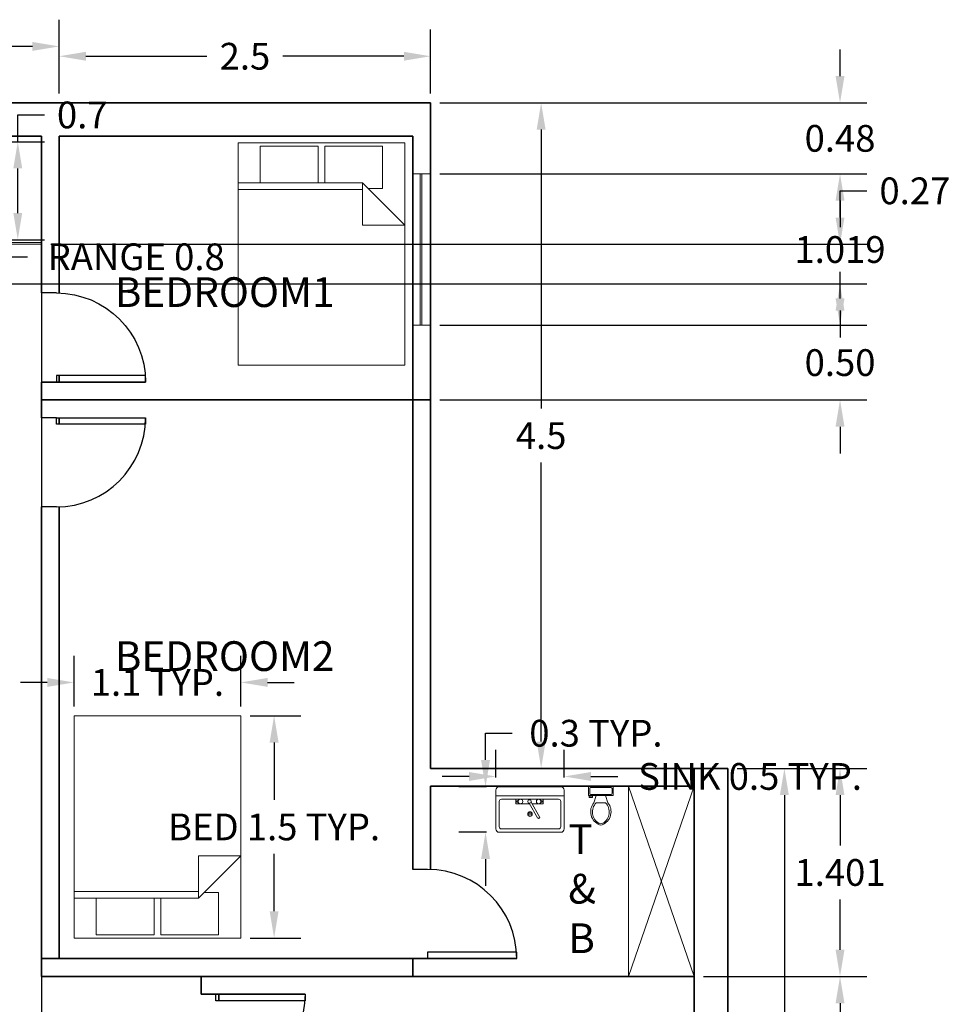
# Model space of a CAD drawing. Units: metres. Extents: x 4.8 to 18.3, y 28.2 to 89.8.
# Tile 4 of 4: x 12 to 18.3, y 36.6 to 43.2. Entities that reach past the tile are written whole.
import ezdxf

# ---------------------------------------------------------------- set-up
doc = ezdxf.new("R2010")
doc.units = ezdxf.units.M
doc.header["$MEASUREMENT"] = 0
doc.layers.get('Defpoints').update_dxf_attribs({"color": 3})
for name, color, linetype, lineweight in [('A-ANNO-DIMS', 2, 'Continuous', 18), ('A-AREA-IDEN', 7, 'Continuous', 25), ('A-DOOR', 3, 'Continuous', 25), ('A-FLOR-CASE', 8, 'Continuous', 18), ('A-FLOR-FIXT', 9, 'Continuous', 18), ('A-FURN', 8, 'Continuous', 18), ('A-GLAZ', 4, 'Continuous', 18), ('A-WALL', 7, 'Continuous', 35)]:
    doc.layers.add(name, color=color, linetype=linetype, lineweight=lineweight)
doc.styles.get("Standard").update_dxf_attribs({"font": 'arial.ttf'})
doc.dimstyles.get("Standard").update_dxf_attribs({"dimtxt": 0.18, "dimasz": 0.18, "dimexe": 0.18, "dimexo": 0.0625, "dimgap": 0.09, "dimtad": 0, "dimtih": 1, "dimtoh": 1, "dimdec": 1, "dimzin": 0, "dimdsep": 46, "dimtxsty": 'Standard', "dimcen": 0.09, "dimadec": 0, "dimazin": 0, "dimtfac": 1, "dimtdec": 1, "dimtofl": 0, "dimtmove": 0, "dimatfit": 3, "dimfxl": 1, "dimtolj": 1, "dimtzin": 0, "dimarcsym": 0})

# ---------------------------------------------------------------- blocks, each defined once
blk = doc.blocks.new('*U3')
for p, q in [((0, 0), (0, -100)), ((600, 0), (600, -100))]:
    blk.add_line(p, q)
blk.add_lwpolyline([(0, 0), (0, 600), (43.75, 600), (43.75, 0)], close=True)
blk.add_arc((0, 0), 600, 0, 90)
blk = doc.blocks.new('Bed - Queen')
for p, q in [((0, -80.00003), (0, 0)), ((0, 0), (59.99999, 0)), ((59.99999, 0), (59.99999, -80.00003)), ((7.99999, -1.2), (28.79998, -1.2)), ((7.99999, -14.4), (7.99999, -1.2)), ((28.79998, -1.2), (28.79998, -14.4)), ((31.19999, -1.2), (51.99999, -1.2)), ((31.19999, -14.4), (31.19999, -1.2)), ((51.99999, -1.2), (51.99999, -16.4)), ((0, -14.4), (44.8, -14.4)), ((44.8, -16.8), (0, -16.8)), ((59.99999, -29.6), (44.8, -14.4)), ((44.8, -14.4), (44.8, -29.6)), ((51.99999, -16.4), (46.79936, -16.4)), ((44.8, -29.6), (59.99999, -29.6)), ((59.99999, -80.00003), (0, -80.00003))]:
    blk.add_line(p, q)
blk = doc.blocks.new('*U14')
for p, q in [((0, 0), (0, 100)), ((600, 0), (600, 100))]:
    blk.add_line(p, q)
blk.add_lwpolyline([(0, 0), (0, -600), (43.75, -600), (43.75, 0)], close=True)
blk.add_arc((0, 0), 600, 270, 0)
blk = doc.blocks.new('Toilet - top')
for p, q in [((-8, -8.5), (-8, -8)), ((-7, -8), (-7, -9.5)), ((-4, -8), (-6, -14)), ((4, -8), (6, -14)), ((9.5, -6), (9.5, -2)), ((-10, -8.5), (-8, -8.5)), ((-10, -9.5), (-10, -8.5)), ((-7, -9.5), (-10, -9.5)), ((4, -14), (-4, -14))]:
    blk.add_line(p, q)
blk.add_lwpolyline([(10.5, -8), (10.5, 0), (-10.5, 0), (-10.5, -8)], close=True)
for points in [[(-9.5, -2), (-9.5, -6)], [(8.5, -1), (-8.5, -1)], [(-8.5, -7), (8.5, -7)]]:
    blk.add_lwpolyline(points)
for centre, radius, start, end in [((-8.62, -1.88), 0.884, 81.8699, 188.1301), ((-8.62, -6.12), 0.884, 171.8699, 278.1301), ((8.62, -1.88), 0.884, 351.8699, 98.1301), ((8.62, -6.12), 0.884, 261.8699, 8.1301), ((3.52, -21.58), 12.17, 141.46911, 247.97143), ((4.2, -21.82), 11.33, 136.36773, 238.94682), ((-3.52, -21.58), 12.17, 292.02843, 38.53071), ((-4.2, -21.82), 11.33, 301.05301, 43.63209), ((0, -27.88), 4, 245.73182, 294.26817), ((0, -29), 4, 254.86053, 285.13947)]:
    blk.add_arc(centre, radius, start, end)
blk = doc.blocks.new('Sink-single - 30 in top')
blk.add_line((-15, -3.999996), (15, -3.999996))
for points in [[(-13.5, 0), (13.5, 0)], [(-15, -18.499996), (-15, -1.5)], [(15, -1.5), (15, -18.499996)], [(-13.5, -17.499996), (-13.5, -6.499996)], [(-12.5, -5.499996), (12.5, -5.499996)], [(13.5, -6.499996), (13.5, -17.499996)], [(13.5, -19.999996), (-13.5, -19.999996)], [(12.5, -18.499996), (-12.5, -18.499996)]]:
    blk.add_lwpolyline(points)
for radius in [1, 0.5]:
    blk.add_circle((0, -11.999996), radius)
for centre, radius, start, end in [((-13.5, -1.5), 1.5, 90, 180), ((13.5, -1.5), 1.5, 0, 90), ((-12.5, -6.499996), 1, 90, 180), ((12.5, -6.499996), 1, 0, 90), ((-13.5, -18.499996), 1.5, 180, 270), ((-12.5, -17.499996), 1, 180, 270), ((12.5, -17.499996), 1, 270, 0), ((13.5, -18.499996), 1.5, 270, 0)]:
    blk.add_arc(centre, radius, start, end)
blk = doc.blocks.new('Faucet - kit sink top')
for p, q in [((-5.5, -0.75), (-5.5, -1.25)), ((-4.94278, -0.75), (-5.5, -0.75)), ((-5.5, -1.25), (-4.94278, -1.25)), ((-0.14775, -1.7441), (3.56698, -8.1782)), ((4.43301, -7.6782), (0.71828, -1.2441)), ((4.94278, -0.75), (5.5, -0.75)), ((5.5, -1.25), (4.94278, -1.25)), ((5.5, -0.75), (5.5, -1.25))]:
    blk.add_line(p, q)
blk.add_lwpolyline([(-0.00587, -2), (-6, -2), (-6, 0), (6, 0), (6, -2), (1.15195, -2)])
for centre, radius in [((-4, -1), 1), ((4, -1), 1), ((0, -1), 0.75)]:
    blk.add_circle(centre, radius)
blk.add_arc((4, -7.9282), 0.5, 210, 30)
blk = doc.blocks.new('*D20')
at = {"layer": 'A-ANNO-DIMS', "color": 0, "lineweight": -2, "transparency": 16777216}
for p, q in [((16.856, 38.1833), (17.355, 38.1833)), ((17.175, 38.0033), (17.175, 35.3333)), ((17.175, 32.2994), (17.175, 34.9694)), ((16.856, 32.1194), (17.355, 32.1194))]:
    blk.add_line(p, q, dxfattribs=at)
at = {"layer": 'A-ANNO-DIMS', "color": 0, "transparency": 16777216}
for points in [[(17.145, 38.0033), (17.205, 38.0033), (17.175, 38.1833)], [(17.145, 32.2994), (17.205, 32.2994), (17.175, 32.1194)]]:
    blk.add_solid(points, dxfattribs=at)
at = {"layer": 'Defpoints', "color": 0, "transparency": 16777216}
for p in [(16.7935, 38.1833), (16.7935, 32.1194), (17.175, 32.1194)]:
    blk.add_point(p, dxfattribs=at)
at = {"layer": 'A-ANNO-DIMS', "color": 0, "transparency": 16777216, "insert": (17.175, 35.1513), "char_height": 0.18, "attachment_point": 5}
blk.add_mtext('\\A1;6.1', dxfattribs=at)
blk = doc.blocks.new('*D21')
at = {"layer": 'A-ANNO-DIMS', "color": 0, "lineweight": -2, "transparency": 16777216}
for p, q in [((14.856, 42.6633), (15.7177, 42.6633)), ((15.5377, 42.4833), (15.5377, 40.6048)), ((15.5377, 38.3633), (15.5377, 40.2417)), ((14.856, 38.1833), (15.7177, 38.1833))]:
    blk.add_line(p, q, dxfattribs=at)
at = {"layer": 'A-ANNO-DIMS', "color": 0, "transparency": 16777216}
for points in [[(15.5077, 42.4833), (15.5677, 42.4833), (15.5377, 42.6633)], [(15.5077, 38.3633), (15.5677, 38.3633), (15.5377, 38.1833)]]:
    blk.add_solid(points, dxfattribs=at)
at = {"layer": 'Defpoints', "color": 0, "transparency": 16777216}
for p in [(14.7935, 42.6633), (14.7935, 38.1833), (15.5377, 38.1833)]:
    blk.add_point(p, dxfattribs=at)
at = {"layer": 'A-ANNO-DIMS', "color": 0, "transparency": 16777216, "insert": (15.5377, 40.4233), "char_height": 0.18, "attachment_point": 5}
blk.add_mtext('\\A1;4.5', dxfattribs=at)
blk = doc.blocks.new('*D22')
at = {"layer": 'A-ANNO-DIMS', "color": 0, "lineweight": -2, "transparency": 16777216}
for p, q in [((6.7935, 42.7258), (6.7935, 43.223)), ((12.2935, 42.7258), (12.2935, 43.223)), ((6.9735, 43.043), (9.289, 43.043)), ((12.1135, 43.043), (9.798, 43.043))]:
    blk.add_line(p, q, dxfattribs=at)
at = {"layer": 'A-ANNO-DIMS', "color": 0, "transparency": 16777216}
for points in [[(6.9735, 43.073), (6.9735, 43.013), (6.7935, 43.043)], [(12.1135, 43.073), (12.1135, 43.013), (12.2935, 43.043)]]:
    blk.add_solid(points, dxfattribs=at)
at = {"layer": 'Defpoints', "color": 0, "transparency": 16777216}
for p in [(12.2935, 43.043), (6.7935, 42.6633), (12.2935, 42.6633)]:
    blk.add_point(p, dxfattribs=at)
at = {"layer": 'A-ANNO-DIMS', "color": 0, "transparency": 16777216, "insert": (9.5435, 43.043), "char_height": 0.18, "attachment_point": 5}
blk.add_mtext('\\A1;5.5', dxfattribs=at)
blk = doc.blocks.new('*D23')
at = {"layer": 'A-ANNO-DIMS', "color": 0, "lineweight": -2, "transparency": 16777216}
for p, q in [((12.2935, 42.7258), (12.2935, 43.1569)), ((14.7935, 42.7255), (14.7935, 43.1569)), ((12.4735, 42.9769), (13.2874, 42.9769)), ((14.6135, 42.9769), (13.7995, 42.9769))]:
    blk.add_line(p, q, dxfattribs=at)
at = {"layer": 'A-ANNO-DIMS', "color": 0, "transparency": 16777216}
for points in [[(12.4735, 43.0069), (12.4735, 42.9469), (12.2935, 42.9769)], [(14.6135, 43.0069), (14.6135, 42.9469), (14.7935, 42.9769)]]:
    blk.add_solid(points, dxfattribs=at)
at = {"layer": 'Defpoints', "color": 0, "transparency": 16777216}
for p in [(14.7935, 42.9769), (12.2935, 42.6633), (14.7935, 42.663)]:
    blk.add_point(p, dxfattribs=at)
at = {"layer": 'A-ANNO-DIMS', "color": 0, "transparency": 16777216, "insert": (13.5435, 42.9769), "char_height": 0.18, "attachment_point": 5}
blk.add_mtext('\\A1;2.5', dxfattribs=at)
blk = doc.blocks.new('*D24')
at = {"layer": 'A-ANNO-DIMS', "color": 0, "lineweight": -2, "transparency": 16777216}
for p, q in [((15.2323, 38.1224), (15.2323, 38.309)), ((15.6928, 38.1224), (15.6928, 38.309)), ((15.0523, 38.129), (14.8723, 38.129)), ((15.8728, 38.129), (16.0528, 38.129))]:
    blk.add_line(p, q, dxfattribs=at)
at = {"layer": 'A-ANNO-DIMS', "color": 0, "transparency": 16777216}
for points in [[(15.0523, 38.159), (15.0523, 38.099), (15.2323, 38.129)], [(15.8728, 38.159), (15.8728, 38.099), (15.6928, 38.129)]]:
    blk.add_solid(points, dxfattribs=at)
at = {"layer": 'Defpoints', "color": 0, "transparency": 16777216}
for p in [(15.6928, 38.129), (15.2323, 38.0599), (15.6928, 38.0599)]:
    blk.add_point(p, dxfattribs=at)
at = {"layer": 'A-ANNO-DIMS', "color": 0, "transparency": 16777216, "insert": (16.9438, 38.129), "char_height": 0.18, "attachment_point": 5}
blk.add_mtext('\\A1;SINK 0.5 TYP.', dxfattribs=at)
blk = doc.blocks.new('*D25')
at = {"layer": 'A-ANNO-DIMS', "color": 0, "lineweight": -2, "transparency": 16777216}
for p, q in [((15.1632, 38.2399), (15.1632, 38.4199)), ((15.1632, 38.4199), (15.3432, 38.4199)), ((15.1698, 38.0599), (14.9832, 38.0599)), ((15.1698, 37.7529), (14.9832, 37.7529)), ((15.1632, 37.5729), (15.1632, 37.3929))]:
    blk.add_line(p, q, dxfattribs=at)
at = {"layer": 'A-ANNO-DIMS', "color": 0, "transparency": 16777216}
for points in [[(15.1332, 38.2399), (15.1932, 38.2399), (15.1632, 38.0599)], [(15.1332, 37.5729), (15.1932, 37.5729), (15.1632, 37.7529)]]:
    blk.add_solid(points, dxfattribs=at)
at = {"layer": 'Defpoints', "color": 0, "transparency": 16777216}
for p in [(15.1632, 38.0599), (15.2323, 38.0599), (15.2323, 37.7529)]:
    blk.add_point(p, dxfattribs=at)
at = {"layer": 'A-ANNO-DIMS', "color": 0, "transparency": 16777216, "insert": (15.9062, 38.4199), "char_height": 0.18, "attachment_point": 5}
blk.add_mtext('\\A1;0.3 TYP.', dxfattribs=at)
blk = doc.blocks.new('*D28')
at = {"layer": 'A-ANNO-DIMS', "color": 0, "lineweight": -2, "transparency": 16777216}
for p, q in [((13.5781, 38.5375), (13.9201, 38.5375)), ((13.7401, 38.3575), (13.7401, 37.9712)), ((13.7401, 37.2211), (13.7401, 37.6074)), ((13.5781, 37.0411), (13.9201, 37.0411))]:
    blk.add_line(p, q, dxfattribs=at)
at = {"layer": 'A-ANNO-DIMS', "color": 0, "transparency": 16777216}
for points in [[(13.7101, 38.3575), (13.7701, 38.3575), (13.7401, 38.5375)], [(13.7101, 37.2211), (13.7701, 37.2211), (13.7401, 37.0411)]]:
    blk.add_solid(points, dxfattribs=at)
at = {"layer": 'Defpoints', "color": 0, "transparency": 16777216}
for p in [(13.5156, 38.5375), (13.5156, 37.0411), (13.7401, 37.0411)]:
    blk.add_point(p, dxfattribs=at)
at = {"layer": 'A-ANNO-DIMS', "color": 0, "transparency": 16777216, "insert": (13.7401, 37.7893), "char_height": 0.18, "attachment_point": 5}
blk.add_mtext('\\A1;BED 1.5 TYP.', dxfattribs=at)
blk = doc.blocks.new('*D29')
at = {"layer": 'A-ANNO-DIMS', "color": 0, "lineweight": -2, "transparency": 16777216}
for p, q in [((12.3933, 38.6), (12.3933, 38.9419)), ((13.5156, 38.6), (13.5156, 38.9419)), ((12.2133, 38.7619), (12.0333, 38.7619)), ((13.6956, 38.7619), (13.8756, 38.7619))]:
    blk.add_line(p, q, dxfattribs=at)
at = {"layer": 'A-ANNO-DIMS', "color": 0, "transparency": 16777216}
for points in [[(12.2133, 38.7919), (12.2133, 38.7319), (12.3933, 38.7619)], [(13.6956, 38.7919), (13.6956, 38.7319), (13.5156, 38.7619)]]:
    blk.add_solid(points, dxfattribs=at)
at = {"layer": 'Defpoints', "color": 0, "transparency": 16777216}
for p in [(13.5156, 38.7619), (12.3933, 38.5375), (13.5156, 38.5375)]:
    blk.add_point(p, dxfattribs=at)
at = {"layer": 'A-ANNO-DIMS', "color": 0, "transparency": 16777216, "insert": (12.9545, 38.7619), "char_height": 0.18, "attachment_point": 5}
blk.add_mtext('\\A1;1.1 TYP.', dxfattribs=at)
blk = doc.blocks.new('*D38')
at = {"layer": 'A-ANNO-DIMS', "color": 0, "lineweight": -2, "transparency": 16777216}
for p, q in [((11.1383, 41.6788), (11.1383, 41.447)), ((11.3183, 41.627), (11.7203, 41.627)), ((11.9003, 41.6788), (11.9003, 41.447)), ((11.9003, 41.627), (12.0803, 41.627))]:
    blk.add_line(p, q, dxfattribs=at)
at = {"layer": 'A-ANNO-DIMS', "color": 0, "transparency": 16777216}
for points in [[(11.3183, 41.657), (11.3183, 41.597), (11.1383, 41.627)], [(11.7203, 41.657), (11.7203, 41.597), (11.9003, 41.627)]]:
    blk.add_solid(points, dxfattribs=at)
at = {"layer": 'Defpoints', "color": 0, "transparency": 16777216}
for p in [(11.1383, 41.7413), (11.9003, 41.7413), (11.9003, 41.627)]:
    blk.add_point(p, dxfattribs=at)
at = {"layer": 'A-ANNO-DIMS', "color": 0, "transparency": 16777216, "insert": (12.8117, 41.627), "char_height": 0.18, "attachment_point": 5}
blk.add_mtext('\\A1;RANGE 0.8', dxfattribs=at)
blk = doc.blocks.new('*D39')
at = {"layer": 'A-ANNO-DIMS', "color": 0, "lineweight": -2, "transparency": 16777216}
for p, q in [((12.0146, 42.4017), (12.0146, 42.5817)), ((12.0146, 42.5817), (12.1946, 42.5817)), ((11.9628, 42.4017), (12.1946, 42.4017)), ((12.0146, 41.9213), (12.0146, 42.2217)), ((11.9628, 41.7413), (12.1946, 41.7413))]:
    blk.add_line(p, q, dxfattribs=at)
at = {"layer": 'A-ANNO-DIMS', "color": 0, "transparency": 16777216}
for points in [[(11.9846, 42.2217), (12.0446, 42.2217), (12.0146, 42.4017)], [(11.9846, 41.9213), (12.0446, 41.9213), (12.0146, 41.7413)]]:
    blk.add_solid(points, dxfattribs=at)
at = {"layer": 'Defpoints', "color": 0, "transparency": 16777216}
for p in [(11.9003, 42.4017), (12.0146, 42.4017), (11.9003, 41.7413)]:
    blk.add_point(p, dxfattribs=at)
at = {"layer": 'A-ANNO-DIMS', "color": 0, "transparency": 16777216, "insert": (12.4485, 42.5817), "char_height": 0.18, "attachment_point": 5}
blk.add_mtext('\\A1;0.7', dxfattribs=at)
blk = doc.blocks.new('*D50')
at = {"layer": 'A-ANNO-DIMS', "color": 0, "lineweight": -2, "transparency": 16777216}
for p, q in [((16.631, 36.7822), (17.7295, 36.7822)), ((17.5495, 36.6022), (17.5495, 35.2892)), ((17.5495, 33.6122), (17.5495, 34.9253)), ((16.631, 33.4322), (17.7295, 33.4322))]:
    blk.add_line(p, q, dxfattribs=at)
at = {"layer": 'A-ANNO-DIMS', "color": 0, "transparency": 16777216}
for points in [[(17.5195, 36.6022), (17.5795, 36.6022), (17.5495, 36.7822)], [(17.5195, 33.6122), (17.5795, 33.6122), (17.5495, 33.4322)]]:
    blk.add_solid(points, dxfattribs=at)
at = {"layer": 'Defpoints', "color": 0, "transparency": 16777216}
for p in [(16.5685, 36.7822), (17.5495, 36.7822), (16.5685, 33.4322)]:
    blk.add_point(p, dxfattribs=at)
at = {"layer": 'A-ANNO-DIMS', "color": 0, "transparency": 16777216, "insert": (17.5495, 35.1072), "char_height": 0.18, "attachment_point": 5}
blk.add_mtext('\\A1;3.35', dxfattribs=at)
blk = doc.blocks.new('*D51')
at = {"layer": 'A-ANNO-DIMS', "color": 0, "lineweight": -2, "transparency": 16777216}
for p, q in [((17.549483, 42.84325), (17.549483, 43.02325)), ((14.855983, 42.66325), (17.729483, 42.66325)), ((14.855983, 42.185448), (17.729483, 42.185448)), ((17.549483, 42.005448), (17.549483, 41.825448))]:
    blk.add_line(p, q, dxfattribs=at)
at = {"layer": 'A-ANNO-DIMS', "color": 0, "transparency": 16777216}
for points in [[(17.519483, 42.84325), (17.579483, 42.84325), (17.549483, 42.66325)], [(17.519483, 42.005448), (17.579483, 42.005448), (17.549483, 42.185448)]]:
    blk.add_solid(points, dxfattribs=at)
at = {"layer": 'Defpoints', "color": 0, "transparency": 16777216}
for p in [(14.793483, 42.66325), (17.549483, 42.66325), (14.793483, 42.185448)]:
    blk.add_point(p, dxfattribs=at)
at = {"layer": 'A-ANNO-DIMS', "color": 0, "transparency": 16777216, "insert": (17.549483, 42.424349), "char_height": 0.18, "attachment_point": 5}
blk.add_mtext('\\A1;0.48', dxfattribs=at)
blk = doc.blocks.new('*D52')
at = {"layer": 'A-ANNO-DIMS', "color": 0, "lineweight": -2, "transparency": 16777216}
for p, q in [((14.856, 42.1854), (17.7295, 42.1854)), ((17.5495, 42.0054), (17.5495, 41.8578)), ((17.5495, 41.3464), (17.5495, 41.494)), ((14.856, 41.1664), (17.7295, 41.1664))]:
    blk.add_line(p, q, dxfattribs=at)
at = {"layer": 'A-ANNO-DIMS', "color": 0, "transparency": 16777216}
for points in [[(17.5195, 42.0054), (17.5795, 42.0054), (17.5495, 42.1854)], [(17.5195, 41.3464), (17.5795, 41.3464), (17.5495, 41.1664)]]:
    blk.add_solid(points, dxfattribs=at)
at = {"layer": 'Defpoints', "color": 0, "transparency": 16777216}
for p in [(14.7935, 42.1854), (17.5495, 42.1854), (14.7935, 41.1664)]:
    blk.add_point(p, dxfattribs=at)
at = {"layer": 'A-ANNO-DIMS', "color": 0, "transparency": 16777216, "insert": (17.5495, 41.6759), "char_height": 0.18, "attachment_point": 5}
blk.add_mtext('\\A1;1.019', dxfattribs=at)
blk = doc.blocks.new('*D53')
at = {"layer": 'A-ANNO-DIMS', "color": 0, "lineweight": -2, "transparency": 16777216}
for p, q in [((17.549483, 41.346372), (17.549483, 41.526372)), ((14.855983, 41.166372), (17.729483, 41.166372)), ((14.855983, 40.66325), (17.729483, 40.66325)), ((17.549483, 40.48325), (17.549483, 40.30325))]:
    blk.add_line(p, q, dxfattribs=at)
at = {"layer": 'A-ANNO-DIMS', "color": 0, "transparency": 16777216}
for points in [[(17.519483, 41.346372), (17.579483, 41.346372), (17.549483, 41.166372)], [(17.519483, 40.48325), (17.579483, 40.48325), (17.549483, 40.66325)]]:
    blk.add_solid(points, dxfattribs=at)
at = {"layer": 'Defpoints', "color": 0, "transparency": 16777216}
for p in [(14.793483, 41.166372), (17.549483, 41.166372), (14.793483, 40.66325)]:
    blk.add_point(p, dxfattribs=at)
at = {"layer": 'A-ANNO-DIMS', "color": 0, "transparency": 16777216, "insert": (17.549483, 40.914811), "char_height": 0.18, "attachment_point": 5}
blk.add_mtext('\\A1;0.50', dxfattribs=at)
blk = doc.blocks.new('*D55')
at = {"layer": 'A-ANNO-DIMS', "color": 0, "lineweight": -2, "transparency": 16777216}
for p, q in [((16.856, 38.1833), (17.7295, 38.1833)), ((17.5495, 38.0033), (17.5495, 37.6647)), ((17.5495, 36.9622), (17.5495, 37.3008)), ((16.631, 36.7822), (17.7295, 36.7822))]:
    blk.add_line(p, q, dxfattribs=at)
at = {"layer": 'A-ANNO-DIMS', "color": 0, "transparency": 16777216}
for points in [[(17.5195, 38.0033), (17.5795, 38.0033), (17.5495, 38.1833)], [(17.5195, 36.9622), (17.5795, 36.9622), (17.5495, 36.7822)]]:
    blk.add_solid(points, dxfattribs=at)
at = {"layer": 'Defpoints', "color": 0, "transparency": 16777216}
for p in [(16.7935, 38.1833), (16.5685, 36.7822), (17.5495, 36.7822)]:
    blk.add_point(p, dxfattribs=at)
at = {"layer": 'A-ANNO-DIMS', "color": 0, "transparency": 16777216, "insert": (17.5495, 37.4827), "char_height": 0.18, "attachment_point": 5}
blk.add_mtext('\\A1;1.401', dxfattribs=at)
blk = doc.blocks.new('*D60')
at = {"layer": 'A-ANNO-DIMS', "color": 0, "lineweight": -2, "transparency": 16777216}
for p, q in [((12.1735, 41.6485), (12.1735, 29.7273)), ((11.5294, 41.3821), (11.5294, 29.7273)), ((11.7094, 29.9073), (11.9935, 29.9073)), ((12.1735, 29.9073), (12.3535, 29.9073))]:
    blk.add_line(p, q, dxfattribs=at)
at = {"layer": 'A-ANNO-DIMS', "color": 0, "transparency": 16777216}
for points in [[(11.7094, 29.9372), (11.7094, 29.8773), (11.5294, 29.9073)], [(11.9935, 29.9372), (11.9935, 29.8773), (12.1735, 29.9073)]]:
    blk.add_solid(points, dxfattribs=at)
at = {"layer": 'Defpoints', "color": 0, "transparency": 16777216}
for p in [(12.1735, 41.711), (11.5294, 41.4446), (12.1735, 29.9073)]:
    blk.add_point(p, dxfattribs=at)
at = {"layer": 'A-ANNO-DIMS', "color": 0, "transparency": 16777216, "insert": (12.7468, 29.9073), "char_height": 0.18, "attachment_point": 5}
blk.add_mtext('\\A1;0.644', dxfattribs=at)
blk = doc.blocks.new('*D61')
at = {"layer": 'A-ANNO-DIMS', "color": 0, "lineweight": -2, "transparency": 16777216}
for p, q in [((17.5495, 41.891), (17.5495, 42.071)), ((17.5495, 42.071), (17.7295, 42.071)), ((12.236, 41.711), (17.7295, 41.711)), ((11.5919, 41.4446), (17.7295, 41.4446)), ((17.5495, 41.2646), (17.5495, 41.0846))]:
    blk.add_line(p, q, dxfattribs=at)
at = {"layer": 'A-ANNO-DIMS', "color": 0, "transparency": 16777216}
for points in [[(17.5195, 41.891), (17.5795, 41.891), (17.5495, 41.711)], [(17.5195, 41.2646), (17.5795, 41.2646), (17.5495, 41.4446)]]:
    blk.add_solid(points, dxfattribs=at)
at = {"layer": 'Defpoints', "color": 0, "transparency": 16777216}
for p in [(12.1735, 41.711), (17.5495, 41.711), (11.5294, 41.4446)]:
    blk.add_point(p, dxfattribs=at)
at = {"layer": 'A-ANNO-DIMS', "color": 0, "transparency": 16777216, "insert": (18.0533, 42.071), "char_height": 0.18, "attachment_point": 5}
blk.add_mtext('\\A1;0.27', dxfattribs=at)

msp = doc.modelspace()

# ---------------------------------------------------------------- linework, layer by layer
at = {"layer": 'A-FLOR-CASE'}
for p, q in [((9.1355, 41.723), (12.1735, 41.723)), ((9.1355, 41.711), (12.1735, 41.711))]:
    msp.add_line(p, q, dxfattribs=at)
at = {"layer": 'A-FLOR-FIXT'}
for p, q in [((16.126, 38.0633), (16.126, 36.7822)), ((16.126, 36.7822), (16.5685, 38.0633)), ((16.126, 38.0633), (16.5685, 36.7822))]:
    msp.add_line(p, q, dxfattribs=at)
at = {"layer": 'A-GLAZ'}
for p, q in [((14.6735, 42.1854), (14.7935, 42.1854)), ((14.7222, 42.1854), (14.7222, 41.1664)), ((14.7335, 42.1854), (14.7274, 42.1854)), ((14.7335, 42.1854), (14.7335, 41.1664)), ((14.6735, 41.1664), (14.7935, 41.1664))]:
    msp.add_line(p, q, dxfattribs=at)
at = {"layer": 'A-WALL'}
for p, q in [((6.7935, 42.6632), (14.7935, 42.6632)), ((14.7935, 38.1833), (14.7935, 42.6632)), ((8.1935, 42.4383), (12.1735, 42.4383)), ((12.1735, 41.711), (12.1735, 42.4383)), ((12.2935, 42.4383), (14.6735, 42.4383)), ((12.2935, 41.383), (12.2935, 42.4383)), ((14.6735, 37.5033), (14.6735, 42.4383)), ((12.1747, 41.3833), (12.1747, 41.711)), ((12.2935, 40.7833), (12.2935, 40.827)), ((12.1735, 40.6632), (12.1735, 40.7833)), ((12.1735, 40.7833), (12.8747, 40.7833)), ((12.1747, 40.7833), (12.1747, 40.6632)), ((12.1735, 40.6632), (14.7935, 40.6632)), ((12.1747, 40.6632), (12.1747, 40.5433)), ((12.2935, 40.4995), (12.2935, 40.5433)), ((12.1747, 39.9433), (12.1747, 36.7833)), ((12.2935, 36.9033), (12.2935, 39.9435)), ((14.7935, 38.1833), (16.7935, 38.1833)), ((16.5685, 38.1833), (16.5685, 33.4322)), ((16.7935, 38.1833), (16.7935, 32.1194)), ((14.7935, 37.5029), (14.7935, 38.0633)), ((14.7935, 38.0633), (16.5685, 38.0633)), ((16.5685, 37.9572), (16.5685, 36.7822)), ((12.1735, 36.9033), (12.1747, 36.9033)), ((12.1747, 36.9033), (15.3735, 36.9033)), ((12.2935, 36.9033), (14.6735, 36.9033)), ((14.6735, 36.7833), (14.6735, 36.9033)), ((14.7735, 36.9033), (14.7935, 36.9033)), ((12.1747, 36.7833), (16.126, 36.7833)), ((13.2485, 36.7833), (13.2485, 36.6633)), ((15.3931, 36.7822), (16.5685, 36.7822)), ((13.2485, 36.6633), (13.9485, 36.6633)), ((13.3685, 36.6633), (13.3685, 36.6195))]:
    msp.add_line(p, q, dxfattribs=at)

# ---------------------------------------------------------------- block references
at = {"layer": 'A-DOOR', "yscale": 0.001, "zscale": 0.001}
for name, p, xscale, rotation in [('*U3', (12.2747, 40.7833), -0.001, 270), ('*U3', (12.2747, 40.5433), 0.001, 270), ('*U14', (14.7735, 36.9033), 0.001, 90), ('*U14', (13.3485, 36.6633), -0.001, 90)]:
    msp.add_blockref(name, p, dxfattribs=dict(at, xscale=xscale, rotation=rotation))
at = {"layer": 'A-FLOR-FIXT'}
for name, p, xscale, yscale, zscale in [('Sink-single - 30 in top', (15.4625, 38.0599), 0.0153508848932381, 0.0153508848932381, 0.0153508848932381), ('Toilet - top', (15.9395, 38.0633), 0.0079224064411582, 0.0079224064411582, 0.0079224064411582), ('Faucet - kit sink top', (15.4594, 37.9755), 0.0153508848932381, 0.0153508848932381, 0.0153508848932381)]:
    msp.add_blockref(name, p, dxfattribs=dict(at, xscale=xscale, yscale=yscale, zscale=zscale))
at = {"layer": 'A-FURN', "xscale": 0.0187047454928596, "yscale": 0.0187047454928596, "zscale": 0.0187047454928596}
msp.add_blockref('Bed - Queen', (13.4972, 42.3945), dxfattribs=at)
at = {"layer": 'A-FURN', "xscale": -0.0187047454928596, "yscale": 0.0187047454928596, "zscale": 0.0187047454928596, "rotation": 180}
msp.add_blockref('Bed - Queen', (12.3933, 37.0411), dxfattribs=at)

# ---------------------------------------------------------------- texts
at = {"layer": 'A-AREA-IDEN', "char_height": 0.2, "attachment_point": 1}
for s, width, insert in [('BEDROOM1', 0.829678, (12.6675, 41.4891)), ('BEDROOM2', 0.829678, (12.6675, 39.039)), ('T & B', 0.334444, (15.7201, 37.8067))]:
    msp.add_mtext_dynamic_manual_height_columns(s, width=width, gutter_width=1, heights=[0], dxfattribs=dict(at, insert=insert))

# ---------------------------------------------------------------- dimensions: what is measured, and where the dimension line sits
at = {"layer": 'A-ANNO-DIMS'}
for base, p1, p2, override, picture, middle in [((12.2935, 43.043), (6.7935, 42.6632), (12.2935, 42.6632), {"dimclrd": 0, "dimclre": 0, "dimclrt": 0}, '*D22', (9.5435, 43.043)), ((14.7935, 42.9769), (12.2935, 42.6632), (14.7935, 42.663), {"dimclrd": 0, "dimclre": 0, "dimclrt": 0}, '*D23', (13.5435, 42.9769)), ((12.1735, 29.9073), (11.5294, 41.4446), (12.1735, 41.711), {"dimdec": 3, "dimlfac": 1, "dimrnd": 0, "dimzin": 0, "dimdsep": 46, "dimlunit": 2}, '*D60', (12.7468, 29.9073))]:
    dim = msp.add_linear_dim(base=base, p1=p1, p2=p2, dimstyle='Standard', override=override, dxfattribs=at)
    dim.commit()
    dim.dimension.update_dxf_attribs({"geometry": picture, "text_midpoint": middle})
for base, p1, p2, override, picture, middle in [((17.5495, 42.6632), (14.7935, 42.1854), (14.7935, 42.6632), {"dimdec": 2, "dimlfac": 1, "dimrnd": 0, "dimzin": 0, "dimdsep": 46, "dimlunit": 2}, '*D51', (17.5495, 42.4243)), ((12.0146, 42.4017), (11.9003, 41.7413), (11.9003, 42.4017), {"dimdec": 1, "dimlfac": 1, "dimrnd": 0, "dimzin": 0, "dimdsep": 46, "dimlunit": 2}, '*D39', (12.4485, 42.5817)), ((15.5377, 38.1833), (14.7935, 42.6632), (14.7935, 38.1833), {"dimclrd": 0, "dimclre": 0, "dimclrt": 0}, '*D21', (15.5377, 40.4233)), ((17.5495, 41.711), (11.5294, 41.4446), (12.1735, 41.711), {"dimdec": 2, "dimlfac": 1, "dimrnd": 0, "dimzin": 0, "dimdsep": 46, "dimlunit": 2}, '*D61', (18.0533, 42.071)), ((17.5495, 42.1854), (14.7935, 41.1664), (14.7935, 42.1854), {"dimdec": 3, "dimlfac": 1, "dimrnd": 0, "dimzin": 0, "dimdsep": 46, "dimlunit": 2}, '*D52', (17.5495, 41.6759)), ((17.5495, 41.1664), (14.7935, 40.6632), (14.7935, 41.1664), {"dimdec": 2, "dimlfac": 1, "dimrnd": 0, "dimzin": 0, "dimdsep": 46, "dimlunit": 2}, '*D53', (17.5495, 40.9148)), ((17.5495, 36.7822), (16.7935, 38.1833), (16.5685, 36.7822), {"dimdec": 3, "dimlfac": 1, "dimrnd": 0, "dimzin": 0, "dimdsep": 46, "dimlunit": 2}, '*D55', (17.5495, 37.4827)), ((17.175, 32.1194), (16.7935, 38.1833), (16.7935, 32.1194), {"dimclrd": 0, "dimclre": 0, "dimclrt": 0}, '*D20', (17.175, 35.1513)), ((17.5495, 36.7822), (16.5685, 33.4322), (16.5685, 36.7822), {"dimdec": 2, "dimlfac": 1, "dimrnd": 0, "dimzin": 0, "dimdsep": 46, "dimlunit": 2}, '*D50', (17.5495, 35.1072))]:
    dim = msp.add_linear_dim(base=base, p1=p1, p2=p2, angle=90, dimstyle='Standard', override=override, dxfattribs=at)
    dim.commit()
    dim.dimension.update_dxf_attribs({"geometry": picture, "text_midpoint": middle})
for base, p1, p2, text, picture, middle in [((11.9003, 41.627), (11.1383, 41.7413), (11.9003, 41.7413), 'RANGE <>', '*D38', (12.8117, 41.627)), ((13.5156, 38.7619), (12.3933, 38.5375), (13.5156, 38.5375), '<> TYP.', '*D29', (12.9545, 38.7619)), ((15.6928, 38.129), (15.2323, 38.0599), (15.6928, 38.0599), 'SINK <> TYP.', '*D24', (16.9438, 38.129))]:
    dim = msp.add_linear_dim(base=base, p1=p1, p2=p2, text=text, dimstyle='Standard', override={"dimdec": 1, "dimlfac": 1, "dimrnd": 0, "dimzin": 0, "dimdsep": 46, "dimlunit": 2}, dxfattribs=at)
    dim.commit()
    dim.dimension.update_dxf_attribs({"geometry": picture, "text_midpoint": middle})
for base, p1, p2, angle, text, picture, middle in [((15.1632, 38.0599), (15.2323, 37.7529), (15.2323, 38.0599), 90, '<> TYP.', '*D25', (15.9062, 38.4199)), ((13.7401, 37.0411), (13.5156, 38.5375), (13.5156, 37.0411), 270, 'BED <> TYP.', '*D28', (13.7401, 37.7893))]:
    dim = msp.add_linear_dim(base=base, p1=p1, p2=p2, angle=angle, text=text, dimstyle='Standard', override={"dimdec": 1, "dimlfac": 1, "dimrnd": 0, "dimzin": 0, "dimdsep": 46, "dimlunit": 2}, dxfattribs=at)
    dim.commit()
    dim.dimension.update_dxf_attribs({"geometry": picture, "text_midpoint": middle})

doc.saveas('drawing.dxf')
